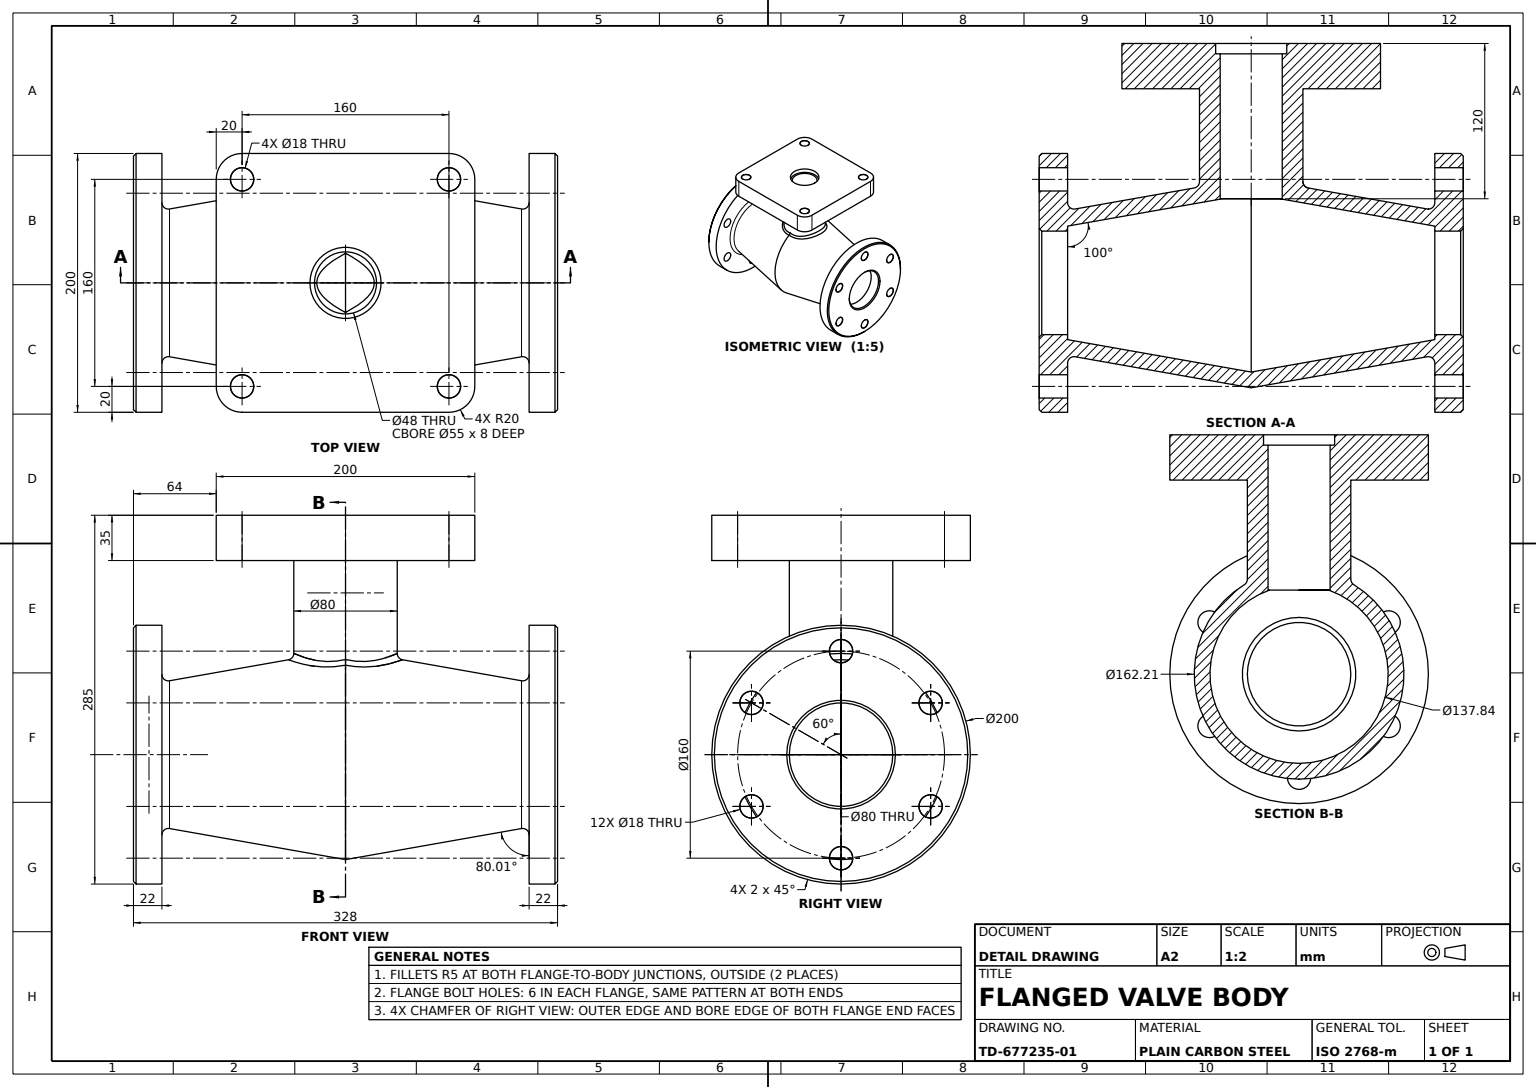
from build123d import *

# Parameters (mm, degrees)
END_FLANGE_PROFILE_200_R            = 100
END_FLANGE_PROFILE_200_R_2          = 40
INLET_FLANGE_DEPTH                  = 22
FLANGE_BOLT_HOLES_6X_18_D           = 18
FLANGE_BOLT_HOLES_6X_18_DEPTH       = 22
FLANGE_BOLT_HOLES_6X_18_CSINK_D     = 18.05
FLANGE_BOLT_HOLES_6X_18_CSINK_ANGLE = 90
BONNET_NECK_80_REACH                = 345.687
BONNET_PAD_AND_NECK_PROFILE_R       = 40
SKETCH7_3_W                         = 200
SKETCH7_3_H                         = 200
SKETCH7_3_R                         = 40
BONNET_PAD_DEPTH                    = 35
BONNET_PAD_CORNER_FILLETS_R20_R     = 20
STEM_BORE_48_C_BORE_55_D            = 48
STEM_BORE_48_C_BORE_55_DEPTH        = 120
STEM_BORE_48_C_BORE_55_CBORE_D      = 55
STEM_BORE_48_C_BORE_55_CBORE_DEPTH  = 8
BONNET_BOLT_HOLES_4X_18_D           = 18
BONNET_BOLT_HOLES_4X_18_CSINK_D     = 18.05
BONNET_BOLT_HOLES_4X_18_CSINK_ANGLE = 90
BODY_BLEND_FILLETS_R5_R             = 5
FLANGE_EDGE_CHAMFERS_2MM_SIZE       = 2


with BuildPart() as part:
    # Body Revolve Profile → Valve Body (revolve)
    with BuildSketch(Plane(origin=(0, 0, 0), x_dir=(0, 0, -1), z_dir=(1, 0, 0)), mode=Mode.PRIVATE) as valve_body_sk:
        Polygon((-164, 40), (0, 68.917624836), (164, 40), (164, 52.185119343), (0, 81.102744179), (-164, 52.185119343), align=None)
    revolve(valve_body_sk.sketch.rotate(Axis((0, 0, 164), (0, 0, -1)), 180), axis=Axis((0, 0, 164), (0, 0, -1)))

    # End Flange Profile _200 → Inlet Flange (add)
    with BuildSketch(Plane.XY.offset(164)):
        Circle(END_FLANGE_PROFILE_200_R)
        Circle(END_FLANGE_PROFILE_200_R_2, mode=Mode.SUBTRACT)
    inlet_flange = extrude(amount=-INLET_FLANGE_DEPTH)

    # Flange Bolt Holes 6x_18
    with Locations(Plane.XY.offset(164)):
        with Locations((-69.282032303, 40), (0, 80), (69.282032303, 40), (69.282032303, -40), (0, -80), (-69.282032303, -40)):
            flange_bolt_holes_6x_18 = CounterSinkHole(FLANGE_BOLT_HOLES_6X_18_D / 2, FLANGE_BOLT_HOLES_6X_18_CSINK_D / 2, depth=FLANGE_BOLT_HOLES_6X_18_DEPTH, counter_sink_angle=FLANGE_BOLT_HOLES_6X_18_CSINK_ANGLE)

    # Outlet Flange Mirror: Inlet Flange, Flange Bolt Holes 6x_18 across plane
    add(inlet_flange.mirror(Plane.XY))
    add(flange_bolt_holes_6x_18.mirror(Plane.XY), mode=Mode.SUBTRACT)

    # Bonnet Pad and Neck Profile → Bonnet Neck _80 (add, up to next)
    with BuildSketch(Plane(origin=(0, 185, 0), x_dir=(1, 0, 0), z_dir=(0, 1, 0)), mode=Mode.PRIVATE) as bonnet_neck_80_sk1:
        with Locations(Location((0, 0, 0), (0, 0, 270))):
            Circle(BONNET_PAD_AND_NECK_PROFILE_R)
    bonnet_neck_80_tool1 = extrude(bonnet_neck_80_sk1.sketch, amount=-BONNET_NECK_80_REACH, mode=Mode.PRIVATE) - part.part
    add(bonnet_neck_80_tool1.solids().sort_by_distance((0, 185, 0))[0])

    # Sketch7_3 → Bonnet Pad (add)
    with BuildSketch(Plane(origin=(0, 185, 0), x_dir=(1, 0, 0), z_dir=(0, 1, 0))):
        Rectangle(SKETCH7_3_W, SKETCH7_3_H)
        with Locations(Location((0, 0, 0), (0, 0, 270))):
            Circle(SKETCH7_3_R, mode=Mode.SUBTRACT)
    extrude(amount=-BONNET_PAD_DEPTH)

    # Bonnet Pad Corner Fillets R20
    bonnet_pad_corner_fillets_r20_edges = [part.edges().sort_by_distance(p)[0] for p in [
        (100, 167.5, -100),
        (100, 167.5, 100),
        (-100, 167.5, 100),
        (-100, 167.5, -100),
    ]]
    fillet(bonnet_pad_corner_fillets_r20_edges, radius=BONNET_PAD_CORNER_FILLETS_R20_R)

    # Stem Bore _48 C-Bore _55
    with Locations(Plane(origin=(0, 185, 0), x_dir=(1, 0, 0), z_dir=(0, 1, 0))):
        with Locations((0, 0)):
            CounterBoreHole(STEM_BORE_48_C_BORE_55_D / 2, STEM_BORE_48_C_BORE_55_CBORE_D / 2, STEM_BORE_48_C_BORE_55_CBORE_DEPTH, depth=STEM_BORE_48_C_BORE_55_DEPTH)

    # Bonnet Bolt Holes 4x_18 (through all)
    with Locations(Plane(origin=(0, 185, 0), x_dir=(1, 0, 0), z_dir=(0, 1, 0))):
        with Locations((-80, -80), (80, -80), (80, 80), (-80, 80)):
            CounterSinkHole(BONNET_BOLT_HOLES_4X_18_D / 2, BONNET_BOLT_HOLES_4X_18_CSINK_D / 2, counter_sink_angle=BONNET_BOLT_HOLES_4X_18_CSINK_ANGLE)

    # Body Blend Fillets R5
    body_blend_fillets_r5_edges = [part.edges().sort_by_distance(p)[0] for p in [
        (0, 74.04966495, -40),
        (28.270667168, 70.668014383, 28.297868784),
        (0, 56.064312918, 142),
        (0, 56.064312918, -142),
    ]]
    fillet(body_blend_fillets_r5_edges, radius=BODY_BLEND_FILLETS_R5_R)

    # Flange Edge Chamfers 2mm
    flange_edge_chamfers_2mm_edges = [part.edges().sort_by_distance(p)[0] for p in [
        (-100, 0, 164),
        (-40, 0, 164),
        (-40, 0, -164),
        (-100, 0, -164),
    ]]
    chamfer(flange_edge_chamfers_2mm_edges, length=FLANGE_EDGE_CHAMFERS_2MM_SIZE)


solid = part.part
